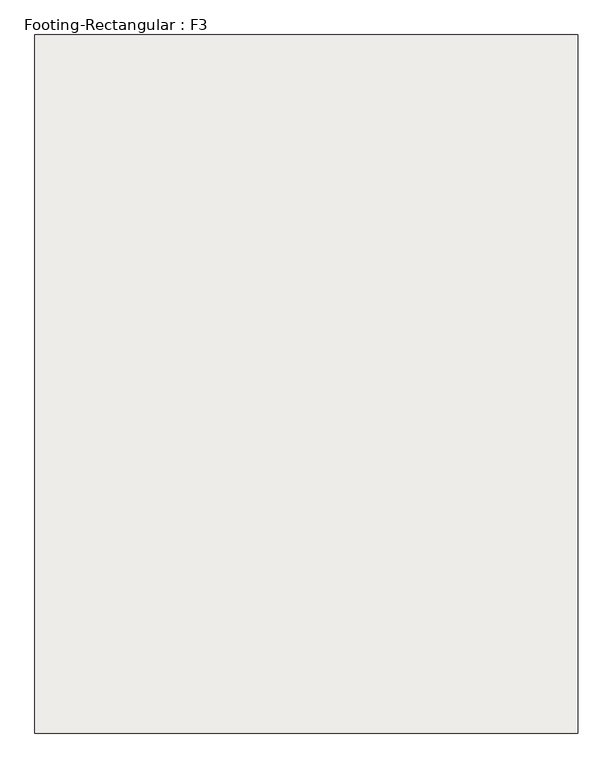
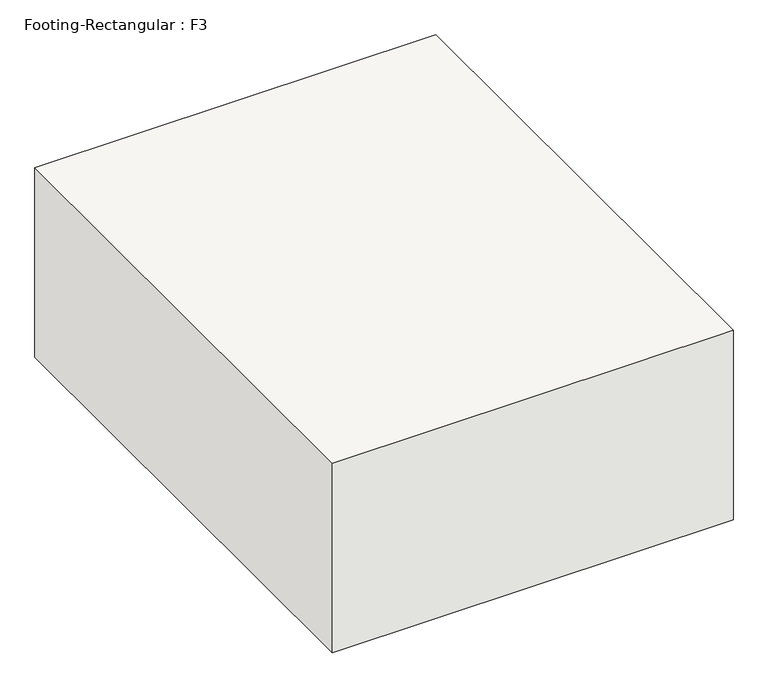
"""IFC4 building model written with IfcOpenShell, lengths in millimetres: slab geometry, Footing-Rectangular : F3."""

from ifc_helpers import new_model, si_unit, frame, origin, place, context, project, spatial, polyline, outline, extrude, source, transform, mapped, element, save


def footing_rectangular_f3_af965022(model_context):
    return source(origin(), model_context, "Body", "SweptSolid", [
        extrude(outline(polyline([(533.4, 685.8), (533.4, -685.8), (-533.4, -685.8), (-533.4, 685.8), (533.4, 685.8)])), frame((0.0, 0.0, -533.4), z_axis=(0.0, 0.0, 1.0), x_axis=(1.0, 0.0, 0.0)), (0.0, 0.0, 1.0), 533.4),
    ])


if __name__ == "__main__":
    model = new_model("IFC4")
    model_context = context("Model", 3, world=origin())
    ifc_project = project(units=[si_unit("LENGTHUNIT", "METRE", prefix="MILLI")], contexts=[model_context])
    site = spatial("IfcSite", under=ifc_project)
    building = spatial("IfcBuilding", under=site)
    placement = place(None, origin())
    footing_rectangular_f3_shape = footing_rectangular_f3_af965022(model_context)
    element("IfcSlab", 1, ObjectType="Footing-Rectangular : F3", at=placement, inside=building, context=model_context, shape_type="MappedRepresentation", body=[
        mapped(footing_rectangular_f3_shape, transform((0.0, 0.0, 0.0), x_axis=(1.0, 0.0, 0.0), y_axis=(0.0, 1.0, 0.0), z_axis=(0.0, 0.0, 1.0))),
    ])
    save(model, "model.ifc")

# Revit data of these elements
# Type "Footing-Rectangular : F3"
#   Width = 1066.8 mm
#   Length = 1371.6 mm
#   Foundation Thickness = 533.4 mm
#   Structural Material [instance default] = Concrete - Cast-in-Place Concrete
#   Assembly Code = ""
# Element 1 (IfcSlab, "Footing-Rectangular : F3")
#   Materials on its faces: "Concrete - Cast-in-Place Concrete"
# Materials
#   "Concrete - Cast-in-Place Concrete": class "Concrete", colour RGB 192 192 192, transparency 0, Cost = 0
